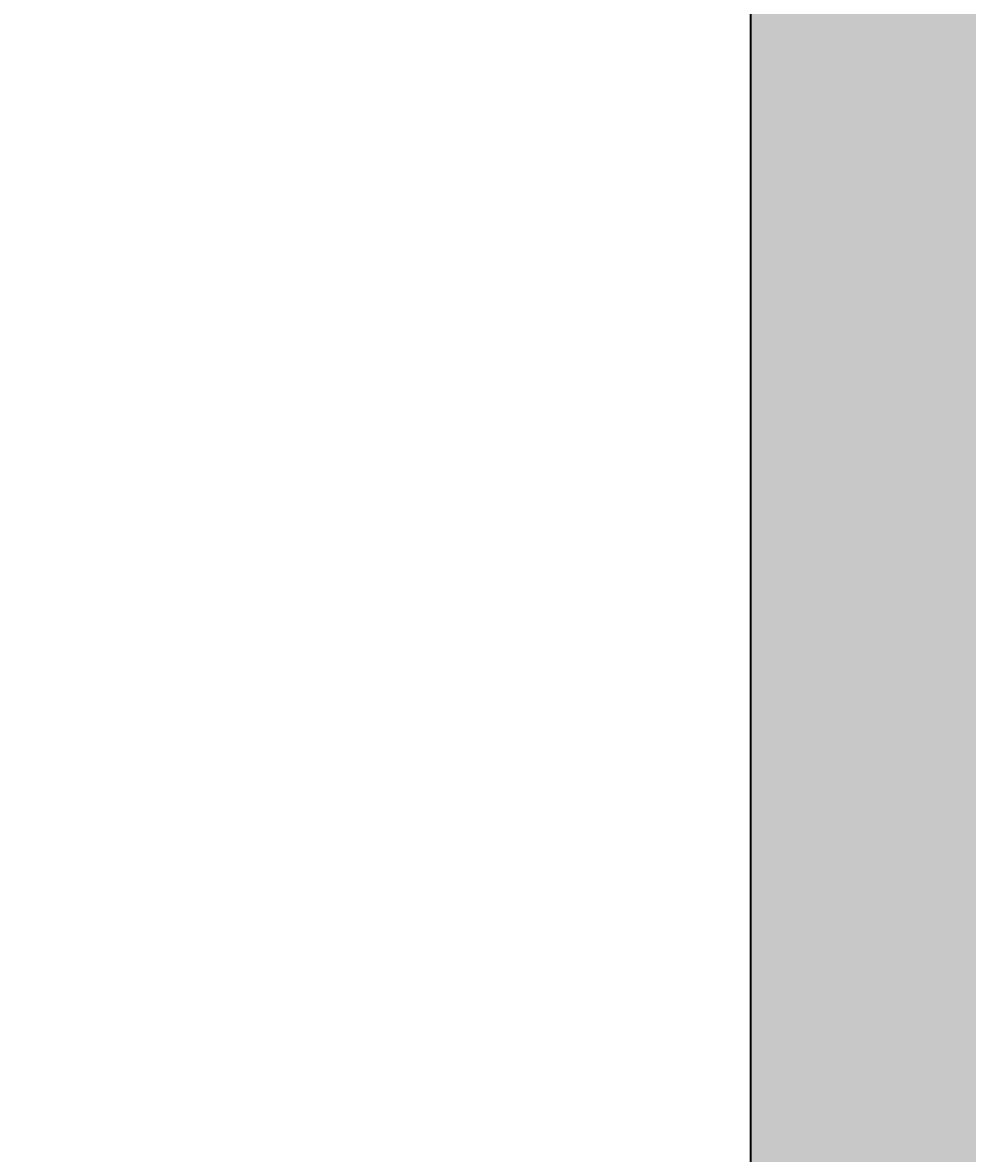
# Model space of a CAD drawing. Units: inches. Extents: x 1998 to 2588, y 1139 to 1977.
# Tile 63 of 134: x 2063 to 2095, y 1779 to 1817. Entities that reach past the tile are written whole.
import ezdxf

# ---------------------------------------------------------------- set-up
doc = ezdxf.new("R2010")
doc.units = ezdxf.units.IN
for name, color, linetype, lineweight in [('A-ANNO-DIMS', 2, 'Continuous', 18), ('A-WALL-PATT', 252, 'Continuous', 13), ('WALL', 200, 'Continuous', 35)]:
    doc.layers.add(name, color=color, linetype=linetype, lineweight=lineweight)
doc.styles.get("Standard").update_dxf_attribs({"font": 'arial.ttf'})
doc.dimstyles.get("Standard").update_dxf_attribs({"dimtxt": 0.18, "dimasz": 0.18, "dimexe": 0.18, "dimexo": 0.0625, "dimgap": 0.09, "dimtad": 0, "dimtih": 1, "dimtoh": 1, "dimdec": 4, "dimzin": 0, "dimdsep": 46, "dimtxsty": 'Standard', "dimcen": 0.09, "dimadec": 0, "dimazin": 0, "dimtfac": 1, "dimtdec": 4, "dimtofl": 0, "dimtmove": 0, "dimatfit": 3, "dimfxl": 1, "dimtolj": 1, "dimtzin": 0, "dimarcsym": 0})

# ---------------------------------------------------------------- blocks, each defined once
blk = doc.blocks.new('*D28')
at = {"layer": 'A-ANNO-DIMS', "color": 0, "lineweight": -2, "transparency": 16777216}
for p, q in [((2059.473, 1759.795), (2059.473, 1977.362)), ((2087.973, 1759.795), (2087.973, 1977.362)), ((2059.653, 1977.182), (2073.397, 1977.182)), ((2087.793, 1977.182), (2074.049, 1977.182))]:
    blk.add_line(p, q, dxfattribs=at)
at = {"layer": 'A-ANNO-DIMS', "color": 0, "transparency": 16777216}
for points in [[(2059.653, 1977.212), (2059.653, 1977.152), (2059.473, 1977.182)], [(2087.793, 1977.212), (2087.793, 1977.152), (2087.973, 1977.182)]]:
    blk.add_solid(points, dxfattribs=at)
at = {"layer": 'Defpoints', "color": 0, "transparency": 16777216}
for p in [(2087.973, 1977.182), (2059.473, 1759.732), (2087.973, 1759.732)]:
    blk.add_point(p, dxfattribs=at)
at = {"layer": 'A-ANNO-DIMS', "color": 0, "transparency": 16777216, "insert": (2073.723, 1977.182), "char_height": 0.18, "attachment_point": 5}
blk.add_mtext('\\A1;28.5', dxfattribs=at)
blk = doc.blocks.new('*D29')
at = {"layer": 'A-ANNO-DIMS', "color": 0, "lineweight": -2, "transparency": 16777216}
for p, q in [((2087.91, 1888.732), (1997.843, 1888.732)), ((1998.023, 1888.552), (1998.023, 1824.414)), ((1998.023, 1759.912), (1998.023, 1824.05)), ((2059.41, 1759.732), (1997.843, 1759.732))]:
    blk.add_line(p, q, dxfattribs=at)
at = {"layer": 'A-ANNO-DIMS', "color": 0, "transparency": 16777216}
for points in [[(1997.993, 1888.552), (1998.053, 1888.552), (1998.023, 1888.732)], [(1997.993, 1759.912), (1998.053, 1759.912), (1998.023, 1759.732)]]:
    blk.add_solid(points, dxfattribs=at)
at = {"layer": 'Defpoints', "color": 0, "transparency": 16777216}
for p in [(1998.023, 1888.732), (2087.973, 1888.732), (2059.473, 1759.732)]:
    blk.add_point(p, dxfattribs=at)
at = {"layer": 'A-ANNO-DIMS', "color": 0, "transparency": 16777216, "insert": (1998.023, 1824.232), "char_height": 0.18, "attachment_point": 5}
blk.add_mtext('\\A1;129', dxfattribs=at)

msp = doc.modelspace()

# ---------------------------------------------------------------- hatches: boundary and pattern name
at = {"layer": 'A-WALL-PATT'}
h = msp.add_hatch(color=256, dxfattribs=at)
h.dxf.hatch_style = 1
h.paths.add_polyline_path([(2222.9729, 1888.7324), (2099.4125, 1888.7324), (2099.4125, 1879.7324), (2222.9729, 1879.7324)])
h.paths.add_polyline_path([(2096.9729, 1868.3278), (2087.9729, 1868.3278), (2087.9729, 1775.637), (2096.9729, 1775.637)])
h.paths.add_polyline_path([(2227.4729, 1868.3278), (2222.9729, 1868.3278), (2222.9729, 1774.3318), (2227.4729, 1774.3318)])
h.paths.add_polyline_path([(2188.3019, 1759.7324), (2138.6074, 1759.7324), (2099.4125, 1759.7324), (2099.4125, 1755.2324), (2176.9729, 1755.2324), (2188.3019, 1755.2324)])
h.paths.add_polyline_path([(2087.9729, 1759.7324), (2059.4729, 1759.7324), (2059.4729, 1702.7324), (2087.9729, 1702.7324), (2087.9729, 1707.2324), (2063.9729, 1707.2324), (2063.9729, 1755.2324), (2087.9729, 1755.2324)])
h.paths.add_polyline_path([(2096.9729, 1755.2324), (2087.9729, 1755.2324), (2087.9729, 1707.2324), (2096.9729, 1707.2324)])
h.paths.add_polyline_path([(2187.0461, 1707.2324), (2105.9729, 1707.2324), (2096.9729, 1707.2324), (2087.9729, 1707.2324), (2087.9729, 1702.7324), (2105.9729, 1702.7324), (2114.9729, 1702.7324), (2187.0461, 1702.7324)])
h.paths.add_polyline_path([(2181.4729, 1719.2028), (2176.9729, 1719.2028), (2176.9729, 1707.2324), (2181.4729, 1707.2324)])
h.paths.add_polyline_path([(2216.0332, 1588.7324), (2114.9729, 1588.7324), (2105.9729, 1588.7324), (2105.9729, 1584.2324), (2216.0332, 1584.2324)])
h.paths.add_polyline_path([(2077.691, 1588.7324), (2061.4729, 1588.7324), (2061.4729, 1584.2324), (2077.691, 1584.2324)])
h.paths.add_polyline_path([(2105.9729, 1588.7324), (2098.0956, 1588.7324), (2098.0956, 1584.2324), (2105.9729, 1584.2324)])
h.paths.add_polyline_path([(2114.9729, 1596.2642), (2110.1012, 1596.2642), (2105.9729, 1596.2642), (2105.9729, 1588.7324), (2114.9729, 1588.7324)])
h.paths.add_polyline_path([(2114.9729, 1584.2324), (2105.9729, 1584.2324), (2105.9729, 1580.249), (2110.1012, 1580.249), (2114.9729, 1580.249)])
h.paths.add_polyline_path([(2114.9729, 1547.7716), (2110.1012, 1547.7716, -0.0318759), (2105.9729, 1548.035), (2105.9729, 1470.2324), (2108.3775, 1470.2324), (2108.3775, 1465.7324), (2186.2943, 1465.7324), (2186.2943, 1470.2324), (2114.9729, 1470.2324)])
h.paths.add_polyline_path([(2227.4729, 1584.2324), (2222.9729, 1584.2324), (2222.9729, 1486.137), (2227.4729, 1486.137)])
h.paths.add_polyline_path([(2295.4138, 1593.2324), (2227.4729, 1593.2324), (2227.4729, 1588.7324), (2295.4138, 1588.7324), (2295.4138, 1591.8729)])
h.paths.add_polyline_path([(2345.9729, 1627.1165), (2341.4729, 1627.1165), (2341.4729, 1593.2324), (2337.2869, 1593.2324), (2337.2869, 1591.8729), (2337.2869, 1588.7324), (2345.9729, 1588.7324)])
h.paths.add_polyline_path([(2291.9729, 1588.7324), (2287.4729, 1588.7324), (2287.4729, 1522.7324), (2291.9729, 1522.7324)])
h.paths.add_polyline_path([(2291.9729, 1522.7324), (2287.4729, 1522.7324), (2227.4729, 1522.7324), (2227.4729, 1518.2324), (2291.9729, 1518.2324)])
h.paths.add_polyline_path([(2295.7347, 1519.5919), (2295.7347, 1522.7324), (2291.9729, 1522.7324), (2291.9729, 1518.2324), (2295.7347, 1518.2324)])
h.paths.add_polyline_path([(2345.9729, 1522.7324), (2337.6078, 1522.7324), (2337.6078, 1519.5919), (2337.6078, 1518.2324), (2341.4729, 1518.2324), (2341.4729, 1488.5616), (2345.9729, 1488.5616)])
h.paths.add_polyline_path([(2345.9729, 1468.1569), (2341.4729, 1468.1569), (2341.4729, 1374.2324), (2227.4729, 1374.2324), (2227.4729, 1369.7324), (2345.9729, 1369.7324)])
h.paths.add_polyline_path([(2345.9729, 1369.7324), (2341.4729, 1369.7324), (2341.4729, 1362.2324), (2345.9729, 1362.2324)])
h.paths.add_polyline_path([(2345.9729, 1317.7324), (2345.9729, 1322.2324), (2341.4729, 1322.2324), (2341.4729, 1285.137), (2345.9729, 1285.137)], flags=17)
h.paths.add_polyline_path([(2356.2096, 1322.2324), (2345.9729, 1322.2324), (2345.9729, 1317.7324), (2356.2096, 1317.7324), (2356.2096, 1319.3088)], flags=17)
h.paths.add_polyline_path([(2393.9729, 1322.2324), (2375.6999, 1322.2324), (2375.6999, 1319.3088, -0.0202458), (2375.636, 1317.7324), (2393.9729, 1317.7324)], flags=17)
h.paths.add_polyline_path([(2398.4729, 1322.2324), (2393.9729, 1322.2324), (2393.9729, 1317.7324), (2393.9729, 1237.7324), (2345.9729, 1237.7324), (2345.9729, 1264.7324), (2341.4729, 1264.7324), (2341.4729, 1228.7324), (2393.9729, 1228.7324), (2482.7412, 1228.7324), (2482.7412, 1237.7324), (2398.4729, 1237.7324), (2398.4729, 1297.1029)])
h.paths.add_polyline_path([(2398.4729, 1362.2324), (2393.9729, 1362.2324), (2393.9729, 1357.7324), (2398.4729, 1357.7324)])
h.paths.add_polyline_path([(2345.9729, 1329.7549), (2341.4729, 1329.7549), (2341.4729, 1322.2324), (2345.9729, 1322.2324)])

# ---------------------------------------------------------------- linework, layer by layer
at = {"layer": 'WALL'}
msp.add_line((2087.9729, 1888.7324), (2087.9729, 1755.2324), dxfattribs=at)

# ---------------------------------------------------------------- dimensions: what is measured, and where the dimension line sits
at = {"layer": 'A-ANNO-DIMS'}
dim = msp.add_linear_dim(base=(2087.9729, 1977.1824), p1=(2059.4729, 1759.7324), p2=(2087.9729, 1759.7324), dimstyle='Standard', override={"dimdec": 1, "dimlfac": 1, "dimrnd": 0, "dimzin": 0, "dimdsep": 46, "dimlunit": 2}, dxfattribs=at)
dim.commit()
dim.dimension.update_dxf_attribs({"geometry": '*D28', "text_midpoint": (2073.7229, 1977.1824)})
dim = msp.add_linear_dim(base=(1998.0229, 1888.7324), p1=(2059.4729, 1759.7324), p2=(2087.9729, 1888.7324), angle=90, dimstyle='Standard', override={"dimdec": 0, "dimlfac": 1, "dimrnd": 0, "dimzin": 0, "dimdsep": 46, "dimlunit": 2}, dxfattribs=at)
dim.commit()
dim.dimension.update_dxf_attribs({"geometry": '*D29', "text_midpoint": (1998.0229, 1824.2324)})

doc.saveas('drawing.dxf')
